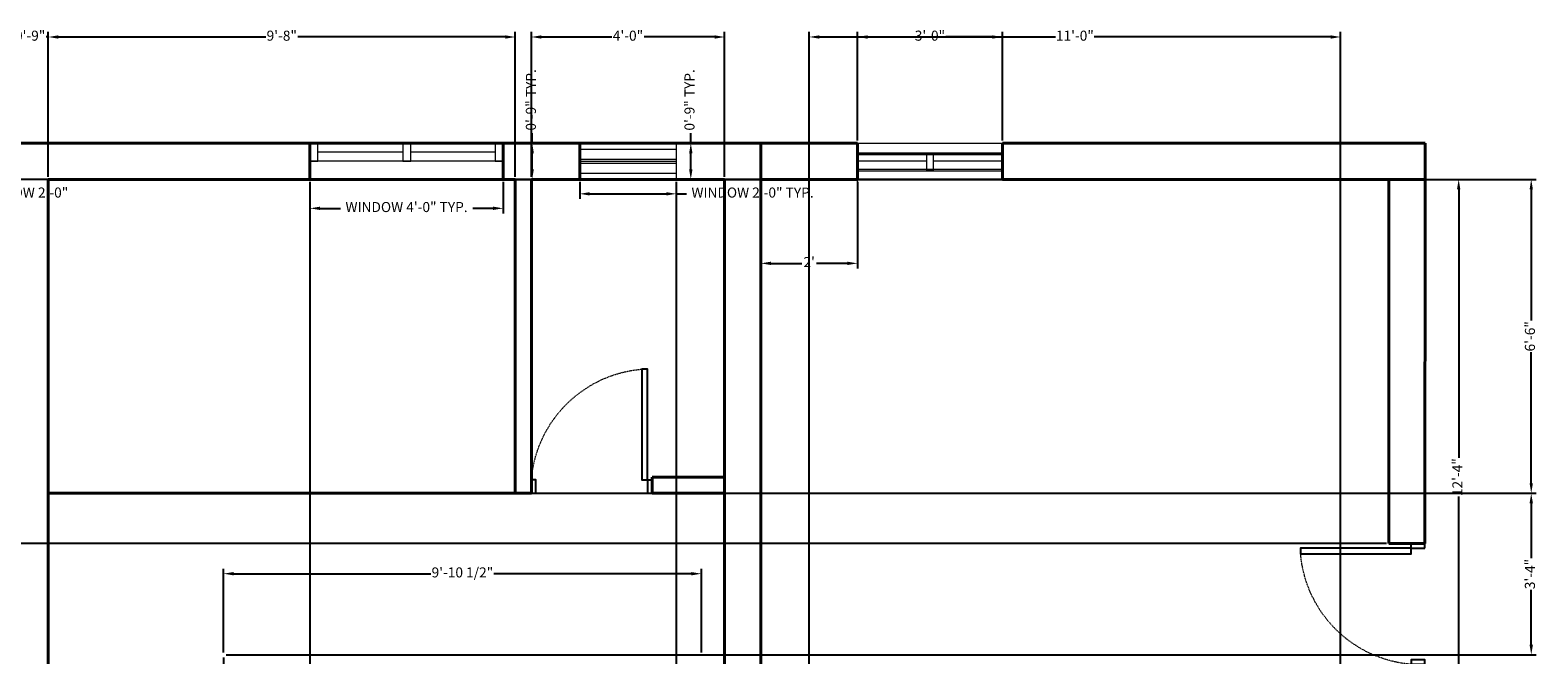
# Model space of a CAD drawing. Units: inches. Extents: x 3502 to 4078, y 3147 to 3541.
# Tile 3 of 3: x 3702 to 4076, y 3386 to 3541. Entities that reach past the tile are written whole.
import ezdxf

# ---------------------------------------------------------------- set-up
doc = ezdxf.new("R2010")
doc.units = ezdxf.units.IN
doc.linetypes.add('HIDDEN4', pattern=[0.09375, 0.0625, -0.03125])
doc.layers.get('0').update_dxf_attribs({"color": 255})
for name, color, linetype, lineweight in [('A-ANNO-DIMS', 2, 'Continuous', 18), ('A-WALL', 7, 'Continuous', 40), ('A-WINDOW', 5, 'Continuous', 15)]:
    doc.layers.add(name, color=color, linetype=linetype, lineweight=lineweight)
doc.layers.add('A-DOOR', color=32, linetype='Continuous', lineweight=25, true_color=0xcd6928)
doc.layers.add('A-DOOR-SWNG', color=32, linetype='HIDDEN4', lineweight=13, true_color=0xcd6928)
doc.styles.get("Standard").update_dxf_attribs({"font": 'arial.ttf'})
doc.dimstyles.new('ISO-25', dxfattribs={"dimtxt": 2.5, "dimasz": 2.5, "dimexe": 1.25, "dimexo": 0.625, "dimtad": 0, "dimlunit": 4, "dimtxsty": 'Standard', "dimcen": 2.5, "dimadec": 0, "dimazin": 0, "dimtfac": 1, "dimtmove": 0, "dimatfit": 3, "dimfxl": 1, "dimarcsym": 0})

# ---------------------------------------------------------------- blocks, each defined once
blk = doc.blocks.new('*D1')
at = {"layer": 'A-ANNO-DIMS', "color": 0, "lineweight": -2, "transparency": 16777216}
for p, q in [((3883.21, 3503.1), (3883.21, 3481.6)), ((3907.21, 3503.1), (3907.21, 3481.6)), ((3885.71, 3482.85), (3893.41, 3482.85)), ((3904.71, 3482.85), (3897.01, 3482.85))]:
    blk.add_line(p, q, dxfattribs=at)
at = {"layer": 'A-ANNO-DIMS', "color": 0, "transparency": 16777216}
for points in [[(3885.71, 3483.26), (3885.71, 3482.43), (3883.21, 3482.85)], [(3904.71, 3483.26), (3904.71, 3482.43), (3907.21, 3482.85)]]:
    blk.add_solid(points, dxfattribs=at)
at = {"layer": 'Defpoints', "color": 0, "transparency": 16777216}
for p in [(3883.21, 3503.72), (3907.21, 3503.72), (3883.21, 3482.85)]:
    blk.add_point(p, dxfattribs=at)
at = {"layer": 'A-ANNO-DIMS', "color": 0, "transparency": 16777216, "insert": (3895.21, 3482.85), "char_height": 2.5, "attachment_point": 5}
blk.add_mtext("2'", dxfattribs=at)
blk = doc.blocks.new('*D3')
at = {"layer": 'A-ANNO-DIMS', "color": 0, "lineweight": -2, "transparency": 16777216}
for p, q in [((4048.83, 3503.72), (4057.8, 3503.72)), ((4056.55, 3501.22), (4056.55, 3434.53)), ((4056.55, 3358.22), (4056.55, 3424.92)), ((4048.83, 3355.72), (4057.8, 3355.72))]:
    blk.add_line(p, q, dxfattribs=at)
at = {"layer": 'A-ANNO-DIMS', "color": 0, "transparency": 16777216}
for points in [[(4056.13, 3501.22), (4056.96, 3501.22), (4056.55, 3503.72)], [(4056.13, 3358.22), (4056.96, 3358.22), (4056.55, 3355.72)]]:
    blk.add_solid(points, dxfattribs=at)
at = {"layer": 'Defpoints', "color": 0, "transparency": 16777216}
for p in [(4048.21, 3503.72), (4048.21, 3355.72), (4056.55, 3355.72)]:
    blk.add_point(p, dxfattribs=at)
at = {"layer": 'A-ANNO-DIMS', "color": 0, "transparency": 16777216, "insert": (4056.55, 3429.72), "char_height": 2.5, "attachment_point": 5, "rotation": 90}
blk.add_mtext('12\'-4"', dxfattribs=at)
blk = doc.blocks.new('A$C63CB6BFC')
at = {"layer": 'A-WALL', "ltscale": 75}
for p, q in [((0, 9), (0, 0)), ((48, 9), (48, 0))]:
    blk.add_line(p, q, dxfattribs=at)
at = {"layer": 'A-WINDOW'}
for p, q in [((48, 9), (0, 9)), ((0, 9), (48, 9)), ((1.99, 4.5), (1.99, 9)), ((23.04, 9), (23.04, 4.5)), ((25.02, 4.5), (25.02, 9)), ((46.01, 9), (46.01, 4.5)), ((48, 4.5), (0, 4.5)), ((0, 4.5), (1.99, 4.5)), ((23.04, 6.75), (1.99, 6.75)), ((23.04, 4.5), (25.02, 4.5)), ((46.01, 6.75), (25.02, 6.75)), ((46.01, 4.5), (48, 4.5)), ((0, 0), (48, 0))]:
    blk.add_line(p, q, dxfattribs=at)
blk = doc.blocks.new('A$C4f83964a')
blk.add_lwpolyline([(0, 9), (24, 9), (24, 0), (0, 0)], close=True)
at = {"layer": 'A-WINDOW'}
for p, q in [((0, 7.5), (24, 7.5)), ((0, 5), (24, 5)), ((0, 4.5), (24, 4.5)), ((0, 4), (24, 4)), ((0, 1.5), (24, 1.5))]:
    blk.add_line(p, q, dxfattribs=at)
blk = doc.blocks.new('dfglkjdg')
at = {"layer": 'A-DOOR'}
for p, q in [((3245.28, 1353.69), (3245.28, 1357.7)), ((3245.28, 1357.7), (3246.64, 1357.7))]:
    blk.add_line(p, q, dxfattribs=at)
for points in [[(3210.73, 1357.7), (3212.09, 1357.7), (3212.09, 1353.69), (3210.73, 1353.69)], [(3210.73, 1353.69), (3210.73, 1357.7)], [(3245.28, 1353.69), (3246.64, 1353.69), (3246.64, 1357.7)]]:
    blk.add_lwpolyline(points, dxfattribs=at)
blk.add_lwpolyline([(3245.28, 1353.69), (3245.28, 1320.78), (3243.61, 1320.78), (3243.61, 1353.69)], close=True, dxfattribs=at)
at = {"layer": 'A-DOOR-SWNG'}
blk.add_arc((3246.64, 1356.69), 36.04, 184.7792, 265.1785, dxfattribs=at)
blk = doc.blocks.new('*D17')
at = {"layer": 'A-ANNO-DIMS', "color": 0, "lineweight": -2, "transparency": 16777216}
for p, q in [((3838.21, 3503.1), (3838.21, 3498.87)), ((3862.21, 3503.1), (3862.21, 3498.87)), ((3840.71, 3500.12), (3859.71, 3500.12)), ((3862.21, 3500.12), (3864.71, 3500.12))]:
    blk.add_line(p, q, dxfattribs=at)
at = {"layer": 'A-ANNO-DIMS', "color": 0, "transparency": 16777216}
for points in [[(3840.71, 3500.54), (3840.71, 3499.71), (3838.21, 3500.12)], [(3859.71, 3500.54), (3859.71, 3499.71), (3862.21, 3500.12)]]:
    blk.add_solid(points, dxfattribs=at)
at = {"layer": 'Defpoints', "color": 0, "transparency": 16777216}
for p in [(3838.21, 3503.72), (3862.21, 3503.72), (3862.21, 3500.12)]:
    blk.add_point(p, dxfattribs=at)
at = {"layer": 'A-ANNO-DIMS', "color": 0, "transparency": 16777216, "insert": (3881.15, 3500.12), "char_height": 2.5, "attachment_point": 5}
blk.add_mtext('WINDOW 2\'-0" TYP.', dxfattribs=at)
blk = doc.blocks.new('*D18')
at = {"layer": 'A-ANNO-DIMS', "color": 0, "lineweight": -2, "transparency": 16777216}
for p, q in [((3865.81, 3512.72), (3865.81, 3515.22)), ((3862.83, 3512.72), (3867.06, 3512.72)), ((3865.81, 3506.22), (3865.81, 3510.22)), ((3862.83, 3503.72), (3867.06, 3503.72))]:
    blk.add_line(p, q, dxfattribs=at)
at = {"layer": 'A-ANNO-DIMS', "color": 0, "transparency": 16777216}
for points in [[(3865.39, 3510.22), (3866.23, 3510.22), (3865.81, 3512.72)], [(3865.39, 3506.22), (3866.23, 3506.22), (3865.81, 3503.72)]]:
    blk.add_solid(points, dxfattribs=at)
at = {"layer": 'Defpoints', "color": 0, "transparency": 16777216}
for p in [(3862.21, 3512.72), (3865.81, 3512.72), (3862.21, 3503.72)]:
    blk.add_point(p, dxfattribs=at)
at = {"layer": 'A-ANNO-DIMS', "color": 0, "transparency": 16777216, "insert": (3865.81, 3523.47), "char_height": 2.5, "attachment_point": 5, "rotation": 90}
blk.add_mtext('0\'-9" TYP.', dxfattribs=at)
blk = doc.blocks.new('*D19')
at = {"layer": 'A-ANNO-DIMS', "color": 0, "lineweight": -2, "transparency": 16777216}
for p, q in [((3771.21, 3503.1), (3771.21, 3495.27)), ((3819.21, 3503.1), (3819.21, 3495.27)), ((3773.71, 3496.52), (3778.77, 3496.52)), ((3816.71, 3496.52), (3811.65, 3496.52))]:
    blk.add_line(p, q, dxfattribs=at)
at = {"layer": 'A-ANNO-DIMS', "color": 0, "transparency": 16777216}
for points in [[(3773.71, 3496.94), (3773.71, 3496.11), (3771.21, 3496.52)], [(3816.71, 3496.94), (3816.71, 3496.11), (3819.21, 3496.52)]]:
    blk.add_solid(points, dxfattribs=at)
at = {"layer": 'Defpoints', "color": 0, "transparency": 16777216}
for p in [(3771.21, 3503.72), (3819.21, 3503.72), (3819.21, 3496.52)]:
    blk.add_point(p, dxfattribs=at)
at = {"layer": 'A-ANNO-DIMS', "color": 0, "transparency": 16777216, "insert": (3795.21, 3496.52), "char_height": 2.5, "attachment_point": 5}
blk.add_mtext('WINDOW 4\'-0" TYP.', dxfattribs=at)
blk = doc.blocks.new('*D20')
at = {"layer": 'A-ANNO-DIMS', "color": 0, "lineweight": -2, "transparency": 16777216}
for p, q in [((3826.41, 3512.72), (3826.41, 3515.22)), ((3819.83, 3512.72), (3827.66, 3512.72)), ((3826.41, 3506.22), (3826.41, 3510.22)), ((3819.83, 3503.72), (3827.66, 3503.72))]:
    blk.add_line(p, q, dxfattribs=at)
at = {"layer": 'A-ANNO-DIMS', "color": 0, "transparency": 16777216}
for points in [[(3825.99, 3510.22), (3826.83, 3510.22), (3826.41, 3512.72)], [(3825.99, 3506.22), (3826.83, 3506.22), (3826.41, 3503.72)]]:
    blk.add_solid(points, dxfattribs=at)
at = {"layer": 'Defpoints', "color": 0, "transparency": 16777216}
for p in [(3819.21, 3512.72), (3826.41, 3512.72), (3819.21, 3503.72)]:
    blk.add_point(p, dxfattribs=at)
at = {"layer": 'A-ANNO-DIMS', "color": 0, "transparency": 16777216, "insert": (3826.41, 3523.47), "char_height": 2.5, "attachment_point": 5, "rotation": 90}
blk.add_mtext('0\'-9" TYP.', dxfattribs=at)
blk = doc.blocks.new('*D23')
at = {"layer": 'A-ANNO-DIMS', "color": 0, "lineweight": -2, "transparency": 16777216}
for p, q in [((3661.21, 3503.1), (3661.21, 3498.87)), ((3685.21, 3503.1), (3685.21, 3498.87)), ((3663.71, 3500.12), (3682.71, 3500.12)), ((3685.21, 3500.12), (3687.71, 3500.12))]:
    blk.add_line(p, q, dxfattribs=at)
at = {"layer": 'A-ANNO-DIMS', "color": 0, "transparency": 16777216}
for points in [[(3663.71, 3500.54), (3663.71, 3499.71), (3661.21, 3500.12)], [(3682.71, 3500.54), (3682.71, 3499.71), (3685.21, 3500.12)]]:
    blk.add_solid(points, dxfattribs=at)
at = {"layer": 'Defpoints', "color": 0, "transparency": 16777216}
for p in [(3661.21, 3503.72), (3685.21, 3503.72), (3685.21, 3500.12)]:
    blk.add_point(p, dxfattribs=at)
at = {"layer": 'A-ANNO-DIMS', "color": 0, "transparency": 16777216, "insert": (3699.86, 3500.12), "char_height": 2.5, "attachment_point": 5}
blk.add_mtext('WINDOW 2\'-0"', dxfattribs=at)
blk = doc.blocks.new('*D32')
at = {"layer": 'A-ANNO-DIMS', "color": 0, "lineweight": -2, "transparency": 16777216}
for p, q in [((3749.73, 3386.19), (3749.73, 3406.98)), ((3752.23, 3405.73), (3801.25, 3405.73)), ((3865.94, 3405.73), (3816.92, 3405.73)), ((3868.44, 3386.19), (3868.44, 3406.98))]:
    blk.add_line(p, q, dxfattribs=at)
at = {"layer": 'A-ANNO-DIMS', "color": 0, "transparency": 16777216}
for points in [[(3752.23, 3406.15), (3752.23, 3405.32), (3749.73, 3405.73)], [(3865.94, 3406.15), (3865.94, 3405.32), (3868.44, 3405.73)]]:
    blk.add_solid(points, dxfattribs=at)
at = {"layer": 'Defpoints', "color": 0, "transparency": 16777216}
for p in [(3868.44, 3405.73), (3749.73, 3385.57), (3868.44, 3385.57)]:
    blk.add_point(p, dxfattribs=at)
at = {"layer": 'A-ANNO-DIMS', "color": 0, "transparency": 16777216, "insert": (3809.08, 3405.73), "char_height": 2.5, "attachment_point": 5}
blk.add_mtext('9\'-10 1/2"', dxfattribs=at)
blk = doc.blocks.new('*D33')
at = {"layer": 'A-ANNO-DIMS', "color": 0, "lineweight": -2, "transparency": 16777216}
for p, q in [((3706.21, 3504.35), (3706.21, 3540.35)), ((3708.71, 3539.1), (3760.26, 3539.1)), ((3819.71, 3539.1), (3768.16, 3539.1)), ((3822.21, 3504.35), (3822.21, 3540.35))]:
    blk.add_line(p, q, dxfattribs=at)
at = {"layer": 'A-ANNO-DIMS', "color": 0, "transparency": 16777216}
for points in [[(3708.71, 3539.51), (3708.71, 3538.68), (3706.21, 3539.1)], [(3819.71, 3539.51), (3819.71, 3538.68), (3822.21, 3539.1)]]:
    blk.add_solid(points, dxfattribs=at)
at = {"layer": 'Defpoints', "color": 0, "transparency": 16777216}
for p in [(3822.21, 3539.1), (3706.21, 3503.72), (3822.21, 3503.72)]:
    blk.add_point(p, dxfattribs=at)
at = {"layer": 'A-ANNO-DIMS', "color": 0, "transparency": 16777216, "insert": (3764.21, 3539.1), "char_height": 2.5, "attachment_point": 5}
blk.add_mtext('9\'-8"', dxfattribs=at)
blk = doc.blocks.new('*D34')
at = {"layer": 'A-ANNO-DIMS', "color": 0, "lineweight": -2, "transparency": 16777216}
for p, q in [((3826.21, 3504.35), (3826.21, 3540.35)), ((3828.71, 3539.1), (3846.21, 3539.1)), ((3871.71, 3539.1), (3854.21, 3539.1)), ((3874.21, 3504.35), (3874.21, 3540.35))]:
    blk.add_line(p, q, dxfattribs=at)
at = {"layer": 'A-ANNO-DIMS', "color": 0, "transparency": 16777216}
for points in [[(3828.71, 3539.51), (3828.71, 3538.68), (3826.21, 3539.1)], [(3871.71, 3539.51), (3871.71, 3538.68), (3874.21, 3539.1)]]:
    blk.add_solid(points, dxfattribs=at)
at = {"layer": 'Defpoints', "color": 0, "transparency": 16777216}
for p in [(3874.21, 3539.1), (3826.21, 3503.72), (3874.21, 3503.72)]:
    blk.add_point(p, dxfattribs=at)
at = {"layer": 'A-ANNO-DIMS', "color": 0, "transparency": 16777216, "insert": (3850.21, 3539.1), "char_height": 2.5, "attachment_point": 5}
blk.add_mtext('4\'-0"', dxfattribs=at)
blk = doc.blocks.new('*D35')
at = {"layer": 'A-ANNO-DIMS', "color": 0, "lineweight": -2, "transparency": 16777216}
for p, q in [((3694.71, 3539.1), (3692.21, 3539.1)), ((3697.21, 3504.35), (3697.21, 3540.35)), ((3697.21, 3539.1), (3697.76, 3539.1)), ((3706.21, 3539.1), (3705.66, 3539.1)), ((3706.21, 3504.35), (3706.21, 3540.35)), ((3708.71, 3539.1), (3711.21, 3539.1))]:
    blk.add_line(p, q, dxfattribs=at)
at = {"layer": 'A-ANNO-DIMS', "color": 0, "transparency": 16777216}
for points in [[(3694.71, 3539.51), (3694.71, 3538.68), (3697.21, 3539.1)], [(3708.71, 3539.51), (3708.71, 3538.68), (3706.21, 3539.1)]]:
    blk.add_solid(points, dxfattribs=at)
at = {"layer": 'Defpoints', "color": 0, "transparency": 16777216}
for p in [(3706.21, 3539.1), (3697.21, 3503.72), (3706.21, 3503.72)]:
    blk.add_point(p, dxfattribs=at)
at = {"layer": 'A-ANNO-DIMS', "color": 0, "transparency": 16777216, "insert": (3701.71, 3539.1), "char_height": 2.5, "attachment_point": 5}
blk.add_mtext('0\'-9"', dxfattribs=at)
blk = doc.blocks.new('*D37')
at = {"layer": 'A-ANNO-DIMS', "color": 0, "lineweight": -2, "transparency": 16777216}
for p, q in [((3907.21, 3513.35), (3907.21, 3540.35)), ((3909.71, 3539.1), (3921.26, 3539.1)), ((3940.71, 3539.1), (3929.16, 3539.1)), ((3943.21, 3513.35), (3943.21, 3540.35))]:
    blk.add_line(p, q, dxfattribs=at)
at = {"layer": 'A-ANNO-DIMS', "color": 0, "transparency": 16777216}
for points in [[(3909.71, 3539.51), (3909.71, 3538.68), (3907.21, 3539.1)], [(3940.71, 3539.51), (3940.71, 3538.68), (3943.21, 3539.1)]]:
    blk.add_solid(points, dxfattribs=at)
at = {"layer": 'Defpoints', "color": 0, "transparency": 16777216}
for p in [(3943.21, 3539.1), (3907.21, 3512.72), (3943.21, 3512.72)]:
    blk.add_point(p, dxfattribs=at)
at = {"layer": 'A-ANNO-DIMS', "color": 0, "transparency": 16777216, "insert": (3925.21, 3539.1), "char_height": 2.5, "attachment_point": 5}
blk.add_mtext('3\'-0"', dxfattribs=at)
blk = doc.blocks.new('*D39')
at = {"layer": 'A-ANNO-DIMS', "color": 0, "lineweight": -2, "transparency": 16777216}
for p, q in [((3706.21, 3503.1), (3706.21, 3149.12)), ((3771.21, 3503.1), (3771.21, 3149.12)), ((3708.71, 3150.37), (3734.76, 3150.37)), ((3768.71, 3150.37), (3742.66, 3150.37))]:
    blk.add_line(p, q, dxfattribs=at)
at = {"layer": 'A-ANNO-DIMS', "color": 0, "transparency": 16777216}
for points in [[(3708.71, 3150.79), (3708.71, 3149.95), (3706.21, 3150.37)], [(3768.71, 3150.79), (3768.71, 3149.95), (3771.21, 3150.37)]]:
    blk.add_solid(points, dxfattribs=at)
at = {"layer": 'Defpoints', "color": 0, "transparency": 16777216}
for p in [(3706.21, 3503.72), (3771.21, 3503.72), (3706.21, 3150.37)]:
    blk.add_point(p, dxfattribs=at)
at = {"layer": 'A-ANNO-DIMS', "color": 0, "transparency": 16777216, "insert": (3738.71, 3150.37), "char_height": 2.5, "attachment_point": 5}
blk.add_mtext('5\'-5"', dxfattribs=at)
blk = doc.blocks.new('*D40')
at = {"layer": 'A-ANNO-DIMS', "color": 0, "lineweight": -2, "transparency": 16777216}
for p, q in [((3862.21, 3503.1), (3862.21, 3149.12)), ((3874.21, 3503.1), (3874.21, 3149.12)), ((3859.71, 3150.37), (3857.21, 3150.37)), ((3862.21, 3150.37), (3864.38, 3150.37)), ((3874.21, 3150.37), (3872.04, 3150.37)), ((3876.71, 3150.37), (3879.21, 3150.37))]:
    blk.add_line(p, q, dxfattribs=at)
at = {"layer": 'A-ANNO-DIMS', "color": 0, "transparency": 16777216}
for points in [[(3859.71, 3150.79), (3859.71, 3149.95), (3862.21, 3150.37)], [(3876.71, 3150.79), (3876.71, 3149.95), (3874.21, 3150.37)]]:
    blk.add_solid(points, dxfattribs=at)
at = {"layer": 'Defpoints', "color": 0, "transparency": 16777216}
for p in [(3862.21, 3503.72), (3874.21, 3503.72), (3874.21, 3150.37)]:
    blk.add_point(p, dxfattribs=at)
at = {"layer": 'A-ANNO-DIMS', "color": 0, "transparency": 16777216, "insert": (3868.21, 3150.37), "char_height": 2.5, "attachment_point": 5}
blk.add_mtext('1\'-0"', dxfattribs=at)
blk = doc.blocks.new('*D42')
at = {"layer": 'A-ANNO-DIMS', "color": 0, "lineweight": -2, "transparency": 16777216}
for p, q in [((3706.83, 3503.72), (4075.82, 3503.72)), ((4074.57, 3501.22), (4074.57, 3468.68)), ((4074.57, 3428.22), (4074.57, 3460.77)), ((3706.83, 3425.72), (4075.82, 3425.72))]:
    blk.add_line(p, q, dxfattribs=at)
at = {"layer": 'A-ANNO-DIMS', "color": 0, "transparency": 16777216}
for points in [[(4074.16, 3501.22), (4074.99, 3501.22), (4074.57, 3503.72)], [(4074.16, 3428.22), (4074.99, 3428.22), (4074.57, 3425.72)]]:
    blk.add_solid(points, dxfattribs=at)
at = {"layer": 'Defpoints', "color": 0, "transparency": 16777216}
for p in [(3706.21, 3503.72), (4074.57, 3503.72), (3706.21, 3425.72)]:
    blk.add_point(p, dxfattribs=at)
at = {"layer": 'A-ANNO-DIMS', "color": 0, "transparency": 16777216, "insert": (4074.57, 3464.72), "char_height": 2.5, "attachment_point": 5, "rotation": 90}
blk.add_mtext('6\'-6"', dxfattribs=at)
blk = doc.blocks.new('*D43')
at = {"layer": 'A-ANNO-DIMS', "color": 0, "lineweight": -2, "transparency": 16777216}
for p, q in [((3895.21, 3186.35), (3895.21, 3540.35)), ((3897.71, 3539.1), (3956.41, 3539.1)), ((4024.71, 3539.1), (3966.01, 3539.1)), ((4027.21, 3186.35), (4027.21, 3540.35))]:
    blk.add_line(p, q, dxfattribs=at)
at = {"layer": 'A-ANNO-DIMS', "color": 0, "transparency": 16777216}
for points in [[(3897.71, 3539.51), (3897.71, 3538.68), (3895.21, 3539.1)], [(4024.71, 3539.51), (4024.71, 3538.68), (4027.21, 3539.1)]]:
    blk.add_solid(points, dxfattribs=at)
at = {"layer": 'Defpoints', "color": 0, "transparency": 16777216}
for p in [(4027.21, 3539.1), (3895.21, 3185.72), (4027.21, 3185.72)]:
    blk.add_point(p, dxfattribs=at)
at = {"layer": 'A-ANNO-DIMS', "color": 0, "transparency": 16777216, "insert": (3961.21, 3539.1), "char_height": 2.5, "attachment_point": 5}
blk.add_mtext('11\'-0"', dxfattribs=at)
blk = doc.blocks.new('*D55')
at = {"layer": 'A-ANNO-DIMS', "color": 0, "lineweight": -2, "transparency": 16777216}
for p, q in [((4038.58, 3503.72), (3504.6, 3503.72)), ((3505.85, 3501.22), (3505.85, 3465.32)), ((3505.85, 3415.71), (3505.85, 3451.62)), ((4038.58, 3413.21), (3504.6, 3413.21))]:
    blk.add_line(p, q, dxfattribs=at)
at = {"layer": 'A-ANNO-DIMS', "color": 0, "transparency": 16777216}
for points in [[(3505.44, 3501.22), (3506.27, 3501.22), (3505.85, 3503.72)], [(3505.44, 3415.71), (3506.27, 3415.71), (3505.85, 3413.21)]]:
    blk.add_solid(points, dxfattribs=at)
at = {"layer": 'Defpoints', "color": 0, "transparency": 16777216}
for p in [(3505.85, 3503.72), (4039.21, 3503.72), (4039.21, 3413.21)]:
    blk.add_point(p, dxfattribs=at)
at = {"layer": 'A-ANNO-DIMS', "color": 0, "transparency": 16777216, "insert": (3505.85, 3458.47), "char_height": 2.5, "attachment_point": 5, "rotation": 90}
blk.add_mtext('7\'-6 1/2"', dxfattribs=at)
blk = doc.blocks.new('*D60')
at = {"layer": 'A-ANNO-DIMS', "color": 0, "lineweight": -2, "transparency": 16777216}
for p, q in [((3706.21, 3425.1), (3706.21, 3149.12)), ((3749.73, 3384.94), (3749.73, 3149.12)), ((3708.71, 3150.37), (3721.11, 3150.37)), ((3747.23, 3150.37), (3734.83, 3150.37))]:
    blk.add_line(p, q, dxfattribs=at)
at = {"layer": 'A-ANNO-DIMS', "color": 0, "transparency": 16777216}
for points in [[(3708.71, 3150.79), (3708.71, 3149.95), (3706.21, 3150.37)], [(3747.23, 3150.79), (3747.23, 3149.95), (3749.73, 3150.37)]]:
    blk.add_solid(points, dxfattribs=at)
at = {"layer": 'Defpoints', "color": 0, "transparency": 16777216}
for p in [(3706.21, 3425.72), (3749.73, 3385.57), (3749.73, 3150.37)]:
    blk.add_point(p, dxfattribs=at)
at = {"layer": 'A-ANNO-DIMS', "color": 0, "transparency": 16777216, "insert": (3727.97, 3150.37), "char_height": 2.5, "attachment_point": 5}
blk.add_mtext('3\'-7 1/2"', dxfattribs=at)
blk = doc.blocks.new('*D61')
at = {"layer": 'A-ANNO-DIMS', "color": 0, "lineweight": -2, "transparency": 16777216}
for p, q in [((3706.83, 3425.72), (4075.82, 3425.72)), ((4074.57, 3423.22), (4074.57, 3409.59)), ((4074.57, 3388.07), (4074.57, 3401.7)), ((3750.36, 3385.57), (4075.82, 3385.57))]:
    blk.add_line(p, q, dxfattribs=at)
at = {"layer": 'A-ANNO-DIMS', "color": 0, "transparency": 16777216}
for points in [[(4074.16, 3423.22), (4074.99, 3423.22), (4074.57, 3425.72)], [(4074.16, 3388.07), (4074.99, 3388.07), (4074.57, 3385.57)]]:
    blk.add_solid(points, dxfattribs=at)
at = {"layer": 'Defpoints', "color": 0, "transparency": 16777216}
for p in [(3706.21, 3425.72), (3749.73, 3385.57), (4074.57, 3385.57)]:
    blk.add_point(p, dxfattribs=at)
at = {"layer": 'A-ANNO-DIMS', "color": 0, "transparency": 16777216, "insert": (4074.57, 3405.65), "char_height": 2.5, "attachment_point": 5, "rotation": 90}
blk.add_mtext('3\'-4"', dxfattribs=at)

msp = doc.modelspace()

# ---------------------------------------------------------------- linework, layer by layer
at = {"layer": 'A-WALL'}
for p, q in [((3819.21, 3503.724), (3819.21, 3512.724)), ((3838.21, 3503.724), (3838.21, 3512.724)), ((3883.21, 3503.724), (3883.21, 3512.724)), ((3907.21, 3503.724), (3907.21, 3512.724)), ((3943.209, 3512.741), (4048.218, 3512.741)), ((3943.21, 3503.724), (3943.21, 3512.724)), ((4048.218, 3512.741), (4048.218, 3503.724)), ((3706.21, 3503.724), (3822.21, 3503.724)), ((3706.21, 3197.724), (3706.21, 3503.724)), ((3822.21, 3425.724), (3822.21, 3503.724)), ((3826.21, 3429.724), (3826.21, 3503.724)), ((3826.21, 3503.724), (3874.21, 3503.724)), ((3874.21, 3197.724), (3874.21, 3503.724)), ((3883.21, 3359.224), (3883.21, 3503.724)), ((4039.21, 3503.724), (4048.21, 3503.724)), ((4048.21, 3503.724), (4048.123, 3413.209)), ((3826.21, 3429.724), (3826.21, 3425.724)), ((3856.21, 3429.724), (3874.21, 3429.724)), ((3856.21, 3429.724), (3856.21, 3425.724)), ((3706.21, 3425.724), (3826.21, 3425.724)), ((3856.21, 3425.724), (3874.21, 3425.724)), ((4039.21, 3413.209), (4048.123, 3413.209))]:
    msp.add_line(p, q, dxfattribs=at)
for points in [[(3685.21, 3512.724), (3907.21, 3512.724)], [(3883.21, 3503.724), (3907.21, 3503.724)], [(3943.21, 3503.724), (4039.21, 3503.724), (4039.21, 3413.209)]]:
    msp.add_lwpolyline(points, dxfattribs=at)
at = {"layer": 'A-WINDOW'}
for p, q in [((3907.21, 3512.741), (3943.209, 3512.741)), ((3907.21, 3501.941), (3907.21, 3512.638)), ((3943.21, 3510.245), (3907.21, 3510.245)), ((3907.21, 3510.245), (3943.21, 3510.245)), ((3943.21, 3509.795), (3907.21, 3509.795)), ((3924.318, 3510.245), (3924.318, 3505.82)), ((3926.102, 3505.82), (3926.102, 3510.245)), ((3943.209, 3512.741), (3943.209, 3505.82)), ((3924.318, 3508.224), (3907.21, 3508.224)), ((3943.21, 3506.203), (3907.21, 3506.203)), ((3907.21, 3505.82), (3943.21, 3505.82)), ((3924.318, 3506.203), (3926.102, 3506.203)), ((3943.21, 3508.224), (3926.102, 3508.224)), ((3907.21, 3503.724), (3943.209, 3503.724))]:
    msp.add_line(p, q, dxfattribs=at)

# ---------------------------------------------------------------- block references
at = {"layer": 'A-DOOR', "xscale": -0.8352314093545642, "yscale": 0.8352314093545642, "zscale": 0.8352314093545642}
for p, rotation in [((1144.51, 4559.718), 180), ((2914.129, 701.51), 270)]:
    msp.add_blockref('dfglkjdg', p, dxfattribs=dict(at, rotation=rotation))
at = {"layer": 'A-WINDOW'}
for name, p in [('A$C63CB6BFC', (3771.21, 3503.724)), ('A$C4f83964a', (3838.21, 3503.724))]:
    msp.add_blockref(name, p, dxfattribs=at)

# ---------------------------------------------------------------- dimensions: what is measured, and where the dimension line sits
at = {"layer": 'A-ANNO-DIMS'}
for base, p1, p2, picture, middle in [((3706.21, 3539.096), (3697.21, 3503.724), (3706.21, 3503.724), '*D35', (3701.71, 3539.096)), ((3822.21, 3539.096), (3706.21, 3503.724), (3822.21, 3503.724), '*D33', (3764.21, 3539.096)), ((3874.21, 3539.096), (3826.21, 3503.724), (3874.21, 3503.724), '*D34', (3850.21, 3539.096)), ((4027.21, 3539.096), (3895.21, 3185.724), (4027.21, 3185.724), '*D43', (3961.21, 3539.096)), ((3943.21, 3539.096), (3907.21, 3512.724), (3943.21, 3512.724), '*D37', (3925.21, 3539.096)), ((3706.21, 3150.369), (3771.21, 3503.724), (3706.21, 3503.724), '*D39', (3738.71, 3150.369)), ((3874.21, 3150.369), (3862.21, 3503.724), (3874.21, 3503.724), '*D40', (3868.21, 3150.369)), ((3749.732, 3150.369), (3706.21, 3425.724), (3749.732, 3385.567), '*D60', (3727.971, 3150.369)), ((3868.435, 3405.734), (3749.732, 3385.567), (3868.435, 3385.567), '*D32', (3809.084, 3405.734))]:
    dim = msp.add_linear_dim(base=base, p1=p1, p2=p2, dimstyle='ISO-25', override={"dimdec": 1, "dimlfac": 1, "dimrnd": 0, "dimzin": 1, "dimdsep": 46, "dimlunit": 4, "dimfrac": 2}, dxfattribs=at)
    dim.commit()
    dim.dimension.update_dxf_attribs({"geometry": picture, "text_midpoint": middle})
for base, p1, p2, picture, middle in [((3826.41, 3512.724), (3819.21, 3503.724), (3819.21, 3512.724), '*D20', (3826.41, 3523.468)), ((3865.81, 3512.724), (3862.21, 3503.724), (3862.21, 3512.724), '*D18', (3865.81, 3523.468))]:
    dim = msp.add_linear_dim(base=base, p1=p1, p2=p2, angle=90, text='<> TYP.', dimstyle='ISO-25', override={"dimdec": 1, "dimlfac": 1, "dimrnd": 0, "dimzin": 1, "dimdsep": 46, "dimlunit": 4, "dimfrac": 2}, dxfattribs=at)
    dim.commit()
    dim.dimension.update_dxf_attribs({"geometry": picture, "text_midpoint": middle})
for base, p1, p2, text, picture, middle in [((3862.21, 3500.124), (3838.21, 3503.724), (3862.21, 3503.724), 'WINDOW <> TYP.', '*D17', (3881.152, 3500.124)), ((3685.21, 3500.124), (3661.21, 3503.724), (3685.21, 3503.724), 'WINDOW <>', '*D23', (3699.856, 3500.124)), ((3819.21, 3496.524), (3771.21, 3503.724), (3819.21, 3503.724), 'WINDOW <> TYP.', '*D19', (3795.21, 3496.524))]:
    dim = msp.add_linear_dim(base=base, p1=p1, p2=p2, text=text, dimstyle='ISO-25', override={"dimdec": 1, "dimlfac": 1, "dimrnd": 0, "dimzin": 1, "dimdsep": 46, "dimlunit": 4, "dimfrac": 2}, dxfattribs=at)
    dim.commit()
    dim.dimension.update_dxf_attribs({"geometry": picture, "text_midpoint": middle})
for base, p1, p2, picture, middle in [((3505.855, 3503.724), (4039.21, 3413.209), (4039.21, 3503.724), '*D55', (3505.855, 3458.467)), ((4074.573, 3503.724), (3706.21, 3425.724), (3706.21, 3503.724), '*D42', (4074.573, 3464.724)), ((4074.573, 3385.567), (3706.21, 3425.724), (3749.732, 3385.567), '*D61', (4074.573, 3405.646))]:
    dim = msp.add_linear_dim(base=base, p1=p1, p2=p2, angle=90, dimstyle='ISO-25', override={"dimdec": 1, "dimlfac": 1, "dimrnd": 0, "dimzin": 1, "dimdsep": 46, "dimlunit": 4, "dimfrac": 2}, dxfattribs=at)
    dim.commit()
    dim.dimension.update_dxf_attribs({"geometry": picture, "text_midpoint": middle})
for p1, p2, distance, picture, middle in [((3907.21, 3503.724), (3883.21, 3503.724), 20.879, '*D1', (3895.21, 3482.845)), ((4048.21, 3503.724), (4048.21, 3355.724), 8.338, '*D3', (4056.548, 3429.724))]:
    dim = msp.add_aligned_dim(p1=p1, p2=p2, distance=distance, dimstyle='ISO-25', override={"dimclrd": 0, "dimclre": 0, "dimclrt": 0}, dxfattribs=at)
    dim.commit()
    dim.dimension.update_dxf_attribs({"geometry": picture, "text_midpoint": middle})

doc.saveas('drawing.dxf')
